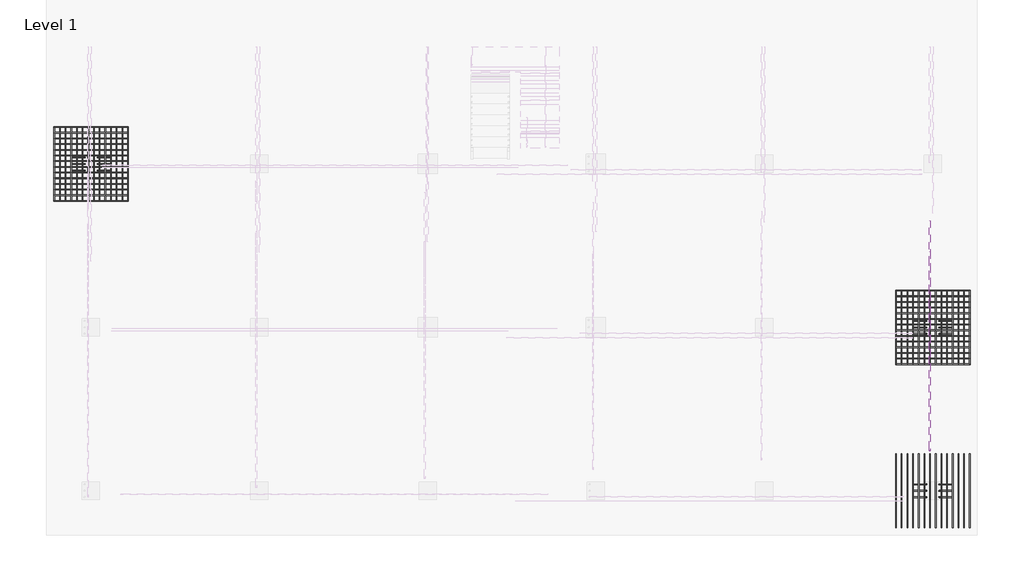
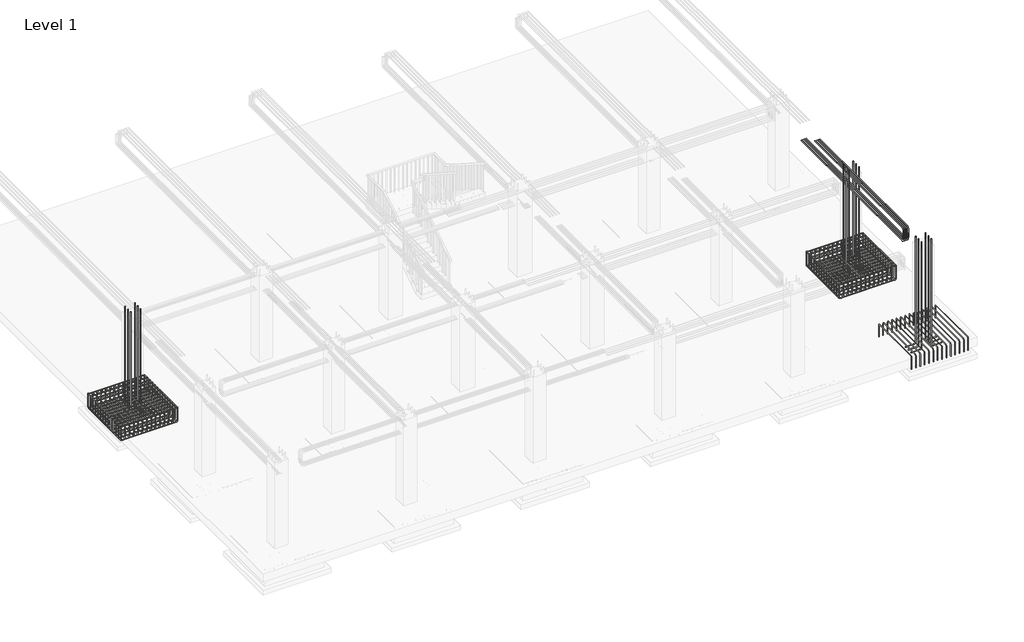
# One storey, part 8 of 17: 19 reinforcing bars.
"""IFC4 building model written with IfcOpenShell, lengths in millimetres."""

from ifc_helpers import new_model, si_unit, point, frame, origin, place, context, project, spatial, polyline, circle_curve, trimmed, segment, composite_curve, source, transform, mapped, element, save
from ifc_brep_helpers import swept_disk

model = new_model("IFC4")

# Units and contexts
model_context = context("Model", 3, world=origin())
ifc_project = project(units=[si_unit("LENGTHUNIT", "METRE", prefix="MILLI")], contexts=[model_context])

# Site, building, storey
site = spatial("IfcSite", under=ifc_project)
building = spatial("IfcBuilding", under=site)
storey = spatial("IfcBuildingStorey", under=building, Name="Level 1", Elevation=0.0)

# Reinforcing bars
placement = place(None, origin())
reinforcing_bar_shape = source(origin(), model_context, "Body", "SolidModel", [
    swept_disk(composite_curve([segment(polyline([(-13686.3632003, 4853.009457, -40.0), (-13686.3632003, 4853.009457, -504.0)]), True, "CONTINUOUS"), segment(trimmed(circle_curve(frame((-13638.3632003, 4853.009457, -504.0), z_axis=(0.0, -1.0, 0.0), x_axis=(-48.0, 0.0, 0.0)), 48.0), [point((-13686.3632003, 4853.009457, -504.0))], [point((-13638.3632003, 4853.009457, -552.0))], True, "CARTESIAN"), True, "CONTINUOUS"), segment(polyline([(-13638.3632003, 4853.009457, -552.0), (-11830.3632003, 4853.009457, -552.0)]), True, "CONTINUOUS"), segment(trimmed(circle_curve(frame((-11830.3632003, 4853.009457, -504.0), z_axis=(0.0, -1.0, 0.0), x_axis=(0.0, 0.0, -48.0)), 48.0), [point((-11830.3632003, 4853.009457, -552.0))], [point((-11782.3632003, 4853.009457, -504.0))], True, "CARTESIAN"), True, "CONTINUOUS"), segment(polyline([(-11782.3632003, 4853.009457, -504.0), (-11782.3632003, 4853.009457, -40.0)]), True, "CONTINUOUS")], self_intersect=False), 8.0),
])
element("IfcReinforcingBar", 1, at=placement, inside=storey, context=model_context, shape_type="MappedRepresentation", body=[
    mapped(reinforcing_bar_shape, transform((0.0, 0.0, 0.0), x_axis=(1.0, 0.0, 0.0), y_axis=(0.0, 1.0, 0.0), z_axis=(0.0, 0.0, 1.0))),
    mapped(reinforcing_bar_shape, transform((0.0, -146.4615385, 0.0), x_axis=(1.0, 0.0, 0.0), y_axis=(0.0, 1.0, 0.0), z_axis=(0.0, 0.0, 1.0))),
    mapped(reinforcing_bar_shape, transform((0.0, -292.9230769, 0.0), x_axis=(1.0, 0.0, 0.0), y_axis=(0.0, 1.0, 0.0), z_axis=(0.0, 0.0, 1.0))),
    mapped(reinforcing_bar_shape, transform((0.0, -439.3846154, 0.0), x_axis=(1.0, 0.0, 0.0), y_axis=(0.0, 1.0, 0.0), z_axis=(0.0, 0.0, 1.0))),
    mapped(reinforcing_bar_shape, transform((0.0, -585.8461538, 0.0), x_axis=(1.0, 0.0, 0.0), y_axis=(0.0, 1.0, 0.0), z_axis=(0.0, 0.0, 1.0))),
    mapped(reinforcing_bar_shape, transform((0.0, -732.3076923, 0.0), x_axis=(1.0, 0.0, 0.0), y_axis=(0.0, 1.0, 0.0), z_axis=(0.0, 0.0, 1.0))),
    mapped(reinforcing_bar_shape, transform((0.0, -878.7692308, 0.0), x_axis=(1.0, 0.0, 0.0), y_axis=(0.0, 1.0, 0.0), z_axis=(0.0, 0.0, 1.0))),
    mapped(reinforcing_bar_shape, transform((0.0, -1025.2307692, 0.0), x_axis=(1.0, 0.0, 0.0), y_axis=(0.0, 1.0, 0.0), z_axis=(0.0, 0.0, 1.0))),
    mapped(reinforcing_bar_shape, transform((0.0, -1171.6923077, 0.0), x_axis=(1.0, 0.0, 0.0), y_axis=(0.0, 1.0, 0.0), z_axis=(0.0, 0.0, 1.0))),
    mapped(reinforcing_bar_shape, transform((0.0, -1318.1538462, 0.0), x_axis=(1.0, 0.0, 0.0), y_axis=(0.0, 1.0, 0.0), z_axis=(0.0, 0.0, 1.0))),
    mapped(reinforcing_bar_shape, transform((0.0, -1464.6153846, 0.0), x_axis=(1.0, 0.0, 0.0), y_axis=(0.0, 1.0, 0.0), z_axis=(0.0, 0.0, 1.0))),
    mapped(reinforcing_bar_shape, transform((0.0, -1611.0769231, 0.0), x_axis=(1.0, 0.0, 0.0), y_axis=(0.0, 1.0, 0.0), z_axis=(0.0, 0.0, 1.0))),
    mapped(reinforcing_bar_shape, transform((0.0, -1757.5384615, 0.0), x_axis=(1.0, 0.0, 0.0), y_axis=(0.0, 1.0, 0.0), z_axis=(0.0, 0.0, 1.0))),
    mapped(reinforcing_bar_shape, transform((0.0, -1904.0, 0.0), x_axis=(1.0, 0.0, 0.0), y_axis=(0.0, 1.0, 0.0), z_axis=(0.0, 0.0, 1.0))),
])
reinforcing_bar_2_shape = source(origin(), model_context, "Body", "SolidModel", [
    swept_disk(composite_curve([segment(polyline([(-13686.3632003, 2949.009457, -504.0), (-13686.3632003, 2949.009457, -96.0)]), True, "CONTINUOUS"), segment(trimmed(circle_curve(frame((-13638.3632003, 2949.009457, -96.0), z_axis=(0.0, 1.0, 0.0), x_axis=(-48.0, 0.0, 0.0)), 48.0), [point((-13686.3632003, 2949.009457, -96.0))], [point((-13638.3632003, 2949.009457, -48.0))], True, "CARTESIAN"), True, "CONTINUOUS"), segment(polyline([(-13638.3632003, 2949.009457, -48.0), (-11830.3632003, 2949.009457, -48.0)]), True, "CONTINUOUS"), segment(trimmed(circle_curve(frame((-11830.3632003, 2949.009457, -96.0), z_axis=(0.0, 1.0, 0.0), x_axis=(0.0, 0.0, 48.0)), 48.0), [point((-11830.3632003, 2949.009457, -48.0))], [point((-11782.3632003, 2949.009457, -96.0))], True, "CARTESIAN"), True, "CONTINUOUS"), segment(polyline([(-11782.3632003, 2949.009457, -96.0), (-11782.3632003, 2949.009457, -504.0)]), True, "CONTINUOUS")], self_intersect=False), 8.0),
])
element("IfcReinforcingBar", 2, at=placement, inside=storey, context=model_context, shape_type="MappedRepresentation", body=[
    mapped(reinforcing_bar_2_shape, transform((0.0, 0.0, 0.0), x_axis=(1.0, 0.0, 0.0), y_axis=(0.0, 1.0, 0.0), z_axis=(0.0, 0.0, 1.0))),
    mapped(reinforcing_bar_2_shape, transform((0.0, 146.4615385, 0.0), x_axis=(1.0, 0.0, 0.0), y_axis=(0.0, 1.0, 0.0), z_axis=(0.0, 0.0, 1.0))),
    mapped(reinforcing_bar_2_shape, transform((0.0, 292.9230769, 0.0), x_axis=(1.0, 0.0, 0.0), y_axis=(0.0, 1.0, 0.0), z_axis=(0.0, 0.0, 1.0))),
    mapped(reinforcing_bar_2_shape, transform((0.0, 439.3846154, 0.0), x_axis=(1.0, 0.0, 0.0), y_axis=(0.0, 1.0, 0.0), z_axis=(0.0, 0.0, 1.0))),
    mapped(reinforcing_bar_2_shape, transform((0.0, 585.8461538, 0.0), x_axis=(1.0, 0.0, 0.0), y_axis=(0.0, 1.0, 0.0), z_axis=(0.0, 0.0, 1.0))),
    mapped(reinforcing_bar_2_shape, transform((0.0, 732.3076923, 0.0), x_axis=(1.0, 0.0, 0.0), y_axis=(0.0, 1.0, 0.0), z_axis=(0.0, 0.0, 1.0))),
    mapped(reinforcing_bar_2_shape, transform((0.0, 878.7692308, 0.0), x_axis=(1.0, 0.0, 0.0), y_axis=(0.0, 1.0, 0.0), z_axis=(0.0, 0.0, 1.0))),
    mapped(reinforcing_bar_2_shape, transform((0.0, 1025.2307692, 0.0), x_axis=(1.0, 0.0, 0.0), y_axis=(0.0, 1.0, 0.0), z_axis=(0.0, 0.0, 1.0))),
    mapped(reinforcing_bar_2_shape, transform((0.0, 1171.6923077, 0.0), x_axis=(1.0, 0.0, 0.0), y_axis=(0.0, 1.0, 0.0), z_axis=(0.0, 0.0, 1.0))),
    mapped(reinforcing_bar_2_shape, transform((0.0, 1318.1538462, 0.0), x_axis=(1.0, 0.0, 0.0), y_axis=(0.0, 1.0, 0.0), z_axis=(0.0, 0.0, 1.0))),
    mapped(reinforcing_bar_2_shape, transform((0.0, 1464.6153846, 0.0), x_axis=(1.0, 0.0, 0.0), y_axis=(0.0, 1.0, 0.0), z_axis=(0.0, 0.0, 1.0))),
    mapped(reinforcing_bar_2_shape, transform((0.0, 1611.0769231, 0.0), x_axis=(1.0, 0.0, 0.0), y_axis=(0.0, 1.0, 0.0), z_axis=(0.0, 0.0, 1.0))),
    mapped(reinforcing_bar_2_shape, transform((0.0, 1757.5384615, 0.0), x_axis=(1.0, 0.0, 0.0), y_axis=(0.0, 1.0, 0.0), z_axis=(0.0, 0.0, 1.0))),
    mapped(reinforcing_bar_2_shape, transform((0.0, 1904.0, 0.0), x_axis=(1.0, 0.0, 0.0), y_axis=(0.0, 1.0, 0.0), z_axis=(0.0, 0.0, 1.0))),
])
reinforcing_bar_3_shape = source(origin(), model_context, "Body", "SolidModel", [
    swept_disk(composite_curve([segment(polyline([(-11782.3632003, 4853.009457, -96.0), (-11782.3632003, 4853.009457, -504.0)]), True, "CONTINUOUS"), segment(trimmed(circle_curve(frame((-11782.3632003, 4805.009457, -504.0), z_axis=(-1.0, 0.0, 0.0), x_axis=(0.0, 48.0, 0.0)), 48.0), [point((-11782.3632003, 4853.009457, -504.0))], [point((-11782.3632003, 4805.009457, -552.0))], True, "CARTESIAN"), True, "CONTINUOUS"), segment(polyline([(-11782.3632003, 4805.009457, -552.0), (-11782.3632003, 2997.009457, -552.0)]), True, "CONTINUOUS"), segment(trimmed(circle_curve(frame((-11782.3632003, 2997.009457, -504.0), z_axis=(-1.0, 0.0, 0.0), x_axis=(0.0, 0.0, -48.0)), 48.0), [point((-11782.3632003, 2997.009457, -552.0))], [point((-11782.3632003, 2949.009457, -504.0))], True, "CARTESIAN"), True, "CONTINUOUS"), segment(polyline([(-11782.3632003, 2949.009457, -504.0), (-11782.3632003, 2949.009457, -96.0)]), True, "CONTINUOUS")], self_intersect=False), 8.0),
])
element("IfcReinforcingBar", 3, at=placement, inside=storey, context=model_context, shape_type="MappedRepresentation", body=[
    mapped(reinforcing_bar_3_shape, transform((0.0, 0.0, 0.0), x_axis=(1.0, 0.0, 0.0), y_axis=(0.0, 1.0, 0.0), z_axis=(0.0, 0.0, 1.0))),
    mapped(reinforcing_bar_3_shape, transform((-146.4615385, 0.0, 0.0), x_axis=(1.0, 0.0, 0.0), y_axis=(0.0, 1.0, 0.0), z_axis=(0.0, 0.0, 1.0))),
    mapped(reinforcing_bar_3_shape, transform((-292.9230769, 0.0, 0.0), x_axis=(1.0, 0.0, 0.0), y_axis=(0.0, 1.0, 0.0), z_axis=(0.0, 0.0, 1.0))),
    mapped(reinforcing_bar_3_shape, transform((-439.3846154, 0.0, 0.0), x_axis=(1.0, 0.0, 0.0), y_axis=(0.0, 1.0, 0.0), z_axis=(0.0, 0.0, 1.0))),
    mapped(reinforcing_bar_3_shape, transform((-585.8461538, 0.0, 0.0), x_axis=(1.0, 0.0, 0.0), y_axis=(0.0, 1.0, 0.0), z_axis=(0.0, 0.0, 1.0))),
    mapped(reinforcing_bar_3_shape, transform((-732.3076923, 0.0, 0.0), x_axis=(1.0, 0.0, 0.0), y_axis=(0.0, 1.0, 0.0), z_axis=(0.0, 0.0, 1.0))),
    mapped(reinforcing_bar_3_shape, transform((-878.7692308, 0.0, 0.0), x_axis=(1.0, 0.0, 0.0), y_axis=(0.0, 1.0, 0.0), z_axis=(0.0, 0.0, 1.0))),
    mapped(reinforcing_bar_3_shape, transform((-1025.2307692, 0.0, 0.0), x_axis=(1.0, 0.0, 0.0), y_axis=(0.0, 1.0, 0.0), z_axis=(0.0, 0.0, 1.0))),
    mapped(reinforcing_bar_3_shape, transform((-1171.6923077, 0.0, 0.0), x_axis=(1.0, 0.0, 0.0), y_axis=(0.0, 1.0, 0.0), z_axis=(0.0, 0.0, 1.0))),
    mapped(reinforcing_bar_3_shape, transform((-1318.1538462, 0.0, 0.0), x_axis=(1.0, 0.0, 0.0), y_axis=(0.0, 1.0, 0.0), z_axis=(0.0, 0.0, 1.0))),
    mapped(reinforcing_bar_3_shape, transform((-1464.6153846, 0.0, 0.0), x_axis=(1.0, 0.0, 0.0), y_axis=(0.0, 1.0, 0.0), z_axis=(0.0, 0.0, 1.0))),
    mapped(reinforcing_bar_3_shape, transform((-1611.0769231, 0.0, 0.0), x_axis=(1.0, 0.0, 0.0), y_axis=(0.0, 1.0, 0.0), z_axis=(0.0, 0.0, 1.0))),
    mapped(reinforcing_bar_3_shape, transform((-1757.5384615, 0.0, 0.0), x_axis=(1.0, 0.0, 0.0), y_axis=(0.0, 1.0, 0.0), z_axis=(0.0, 0.0, 1.0))),
    mapped(reinforcing_bar_3_shape, transform((-1904.0, 0.0, 0.0), x_axis=(1.0, 0.0, 0.0), y_axis=(0.0, 1.0, 0.0), z_axis=(0.0, 0.0, 1.0))),
])
reinforcing_bar_4_shape = source(origin(), model_context, "Body", "SolidModel", [
    swept_disk(composite_curve([segment(polyline([(-13686.3632003, 4853.009457, -504.0), (-13686.3632003, 4853.009457, -96.0)]), True, "CONTINUOUS"), segment(trimmed(circle_curve(frame((-13686.3632003, 4805.009457, -96.0), z_axis=(1.0, 0.0, 0.0), x_axis=(0.0, 48.0, 0.0)), 48.0), [point((-13686.3632003, 4853.009457, -96.0))], [point((-13686.3632003, 4805.009457, -48.0))], True, "CARTESIAN"), True, "CONTINUOUS"), segment(polyline([(-13686.3632003, 4805.009457, -48.0), (-13686.3632003, 2997.009457, -48.0)]), True, "CONTINUOUS"), segment(trimmed(circle_curve(frame((-13686.3632003, 2997.009457, -96.0), z_axis=(1.0, 0.0, 0.0), x_axis=(0.0, 0.0, 48.0)), 48.0), [point((-13686.3632003, 2997.009457, -48.0))], [point((-13686.3632003, 2949.009457, -96.0))], True, "CARTESIAN"), True, "CONTINUOUS"), segment(polyline([(-13686.3632003, 2949.009457, -96.0), (-13686.3632003, 2949.009457, -504.0)]), True, "CONTINUOUS")], self_intersect=False), 8.0),
])
element("IfcReinforcingBar", 4, at=placement, inside=storey, context=model_context, shape_type="MappedRepresentation", body=[
    mapped(reinforcing_bar_4_shape, transform((0.0, 0.0, 0.0), x_axis=(1.0, 0.0, 0.0), y_axis=(0.0, 1.0, 0.0), z_axis=(0.0, 0.0, 1.0))),
    mapped(reinforcing_bar_4_shape, transform((146.4615385, 0.0, 0.0), x_axis=(1.0, 0.0, 0.0), y_axis=(0.0, 1.0, 0.0), z_axis=(0.0, 0.0, 1.0))),
    mapped(reinforcing_bar_4_shape, transform((292.9230769, 0.0, 0.0), x_axis=(1.0, 0.0, 0.0), y_axis=(0.0, 1.0, 0.0), z_axis=(0.0, 0.0, 1.0))),
    mapped(reinforcing_bar_4_shape, transform((439.3846154, 0.0, 0.0), x_axis=(1.0, 0.0, 0.0), y_axis=(0.0, 1.0, 0.0), z_axis=(0.0, 0.0, 1.0))),
    mapped(reinforcing_bar_4_shape, transform((585.8461538, 0.0, 0.0), x_axis=(1.0, 0.0, 0.0), y_axis=(0.0, 1.0, 0.0), z_axis=(0.0, 0.0, 1.0))),
    mapped(reinforcing_bar_4_shape, transform((732.3076923, 0.0, 0.0), x_axis=(1.0, 0.0, 0.0), y_axis=(0.0, 1.0, 0.0), z_axis=(0.0, 0.0, 1.0))),
    mapped(reinforcing_bar_4_shape, transform((878.7692308, 0.0, 0.0), x_axis=(1.0, 0.0, 0.0), y_axis=(0.0, 1.0, 0.0), z_axis=(0.0, 0.0, 1.0))),
    mapped(reinforcing_bar_4_shape, transform((1025.2307692, 0.0, 0.0), x_axis=(1.0, 0.0, 0.0), y_axis=(0.0, 1.0, 0.0), z_axis=(0.0, 0.0, 1.0))),
    mapped(reinforcing_bar_4_shape, transform((1171.6923077, 0.0, 0.0), x_axis=(1.0, 0.0, 0.0), y_axis=(0.0, 1.0, 0.0), z_axis=(0.0, 0.0, 1.0))),
    mapped(reinforcing_bar_4_shape, transform((1318.1538462, 0.0, 0.0), x_axis=(1.0, 0.0, 0.0), y_axis=(0.0, 1.0, 0.0), z_axis=(0.0, 0.0, 1.0))),
    mapped(reinforcing_bar_4_shape, transform((1464.6153846, 0.0, 0.0), x_axis=(1.0, 0.0, 0.0), y_axis=(0.0, 1.0, 0.0), z_axis=(0.0, 0.0, 1.0))),
    mapped(reinforcing_bar_4_shape, transform((1611.0769231, 0.0, 0.0), x_axis=(1.0, 0.0, 0.0), y_axis=(0.0, 1.0, 0.0), z_axis=(0.0, 0.0, 1.0))),
    mapped(reinforcing_bar_4_shape, transform((1757.5384615, 0.0, 0.0), x_axis=(1.0, 0.0, 0.0), y_axis=(0.0, 1.0, 0.0), z_axis=(0.0, 0.0, 1.0))),
    mapped(reinforcing_bar_4_shape, transform((1904.0, 0.0, 0.0), x_axis=(1.0, 0.0, 0.0), y_axis=(0.0, 1.0, 0.0), z_axis=(0.0, 0.0, 1.0))),
])
reinforcing_bar_5_shape = source(origin(), model_context, "Body", "SolidModel", [
    swept_disk(composite_curve([segment(polyline([(-13246.9785849, 4066.509457, -550.0), (-12949.8632003, 4066.509457, -550.0)]), True, "CONTINUOUS"), segment(trimmed(circle_curve(frame((-12949.8632003, 4066.509457, -500.0), z_axis=(0.0, -1.0, 0.0), x_axis=(0.0, 0.0, -50.0)), 50.0), [point((-12949.8632003, 4066.509457, -550.0))], [point((-12899.8632003, 4066.509457, -500.0))], True, "CARTESIAN"), True, "CONTINUOUS"), segment(polyline([(-12899.8632003, 4066.509457, -500.0), (-12899.8632003, 4066.509457, 3260.0)]), True, "CONTINUOUS")], self_intersect=False), 10.0),
])
element("IfcReinforcingBar", 5, at=placement, inside=storey, context=model_context, shape_type="MappedRepresentation", body=[
    mapped(reinforcing_bar_5_shape, transform((0.0, 0.0, 0.0), x_axis=(1.0, 0.0, 0.0), y_axis=(0.0, 1.0, 0.0), z_axis=(0.0, 0.0, 1.0))),
    mapped(reinforcing_bar_5_shape, transform((0.0, -165.5, 0.0), x_axis=(1.0, 0.0, 0.0), y_axis=(0.0, 1.0, 0.0), z_axis=(0.0, 0.0, 1.0))),
    mapped(reinforcing_bar_5_shape, transform((0.0, -331.0, 0.0), x_axis=(1.0, 0.0, 0.0), y_axis=(0.0, 1.0, 0.0), z_axis=(0.0, 0.0, 1.0))),
])
reinforcing_bar_6_shape = source(origin(), model_context, "Body", "SolidModel", [
    swept_disk(composite_curve([segment(polyline([(-12221.7478157, 3735.509457, -550.0), (-12518.8632003, 3735.509457, -550.0)]), True, "CONTINUOUS"), segment(trimmed(circle_curve(frame((-12518.8632003, 3735.509457, -500.0), z_axis=(0.0, 1.0, 0.0), x_axis=(0.0, 0.0, -50.0)), 50.0), [point((-12518.8632003, 3735.509457, -550.0))], [point((-12568.8632003, 3735.509457, -500.0))], True, "CARTESIAN"), True, "CONTINUOUS"), segment(polyline([(-12568.8632003, 3735.509457, -500.0), (-12568.8632003, 3735.509457, 3260.0)]), True, "CONTINUOUS")], self_intersect=False), 10.0),
])
element("IfcReinforcingBar", 6, at=placement, inside=storey, context=model_context, shape_type="MappedRepresentation", body=[
    mapped(reinforcing_bar_6_shape, transform((0.0, 0.0, 0.0), x_axis=(1.0, 0.0, 0.0), y_axis=(0.0, 1.0, 0.0), z_axis=(0.0, 0.0, 1.0))),
    mapped(reinforcing_bar_6_shape, transform((0.0, 165.5, 0.0), x_axis=(1.0, 0.0, 0.0), y_axis=(0.0, 1.0, 0.0), z_axis=(0.0, 0.0, 1.0))),
    mapped(reinforcing_bar_6_shape, transform((0.0, 331.0, 0.0), x_axis=(1.0, 0.0, 0.0), y_axis=(0.0, 1.0, 0.0), z_axis=(0.0, 0.0, 1.0))),
])
reinforcing_bar_7_shape = source(origin(), model_context, "Body", "SolidModel", [
    swept_disk(composite_curve([segment(polyline([(8038.6367997, 636.009457, -40.0), (8038.6367997, 636.009457, -504.0)]), True, "CONTINUOUS"), segment(trimmed(circle_curve(frame((8086.6367997, 636.009457, -504.0), z_axis=(0.0, -1.0, 0.0), x_axis=(-48.0, 0.0, 0.0)), 48.0), [point((8038.6367997, 636.009457, -504.0))], [point((8086.6367997, 636.009457, -552.0))], True, "CARTESIAN"), True, "CONTINUOUS"), segment(polyline([(8086.6367997, 636.009457, -552.0), (9894.6367997, 636.009457, -552.0)]), True, "CONTINUOUS"), segment(trimmed(circle_curve(frame((9894.6367997, 636.009457, -504.0), z_axis=(0.0, -1.0, 0.0), x_axis=(0.0, 0.0, -48.0)), 48.0), [point((9894.6367997, 636.009457, -552.0))], [point((9942.6367997, 636.009457, -504.0))], True, "CARTESIAN"), True, "CONTINUOUS"), segment(polyline([(9942.6367997, 636.009457, -504.0), (9942.6367997, 636.009457, -40.0)]), True, "CONTINUOUS")], self_intersect=False), 8.0),
])
element("IfcReinforcingBar", 7, at=placement, inside=storey, context=model_context, shape_type="MappedRepresentation", body=[
    mapped(reinforcing_bar_7_shape, transform((0.0, 0.0, 0.0), x_axis=(1.0, 0.0, 0.0), y_axis=(0.0, 1.0, 0.0), z_axis=(0.0, 0.0, 1.0))),
    mapped(reinforcing_bar_7_shape, transform((0.0, -146.4615385, 0.0), x_axis=(1.0, 0.0, 0.0), y_axis=(0.0, 1.0, 0.0), z_axis=(0.0, 0.0, 1.0))),
    mapped(reinforcing_bar_7_shape, transform((0.0, -292.9230769, 0.0), x_axis=(1.0, 0.0, 0.0), y_axis=(0.0, 1.0, 0.0), z_axis=(0.0, 0.0, 1.0))),
    mapped(reinforcing_bar_7_shape, transform((0.0, -439.3846154, 0.0), x_axis=(1.0, 0.0, 0.0), y_axis=(0.0, 1.0, 0.0), z_axis=(0.0, 0.0, 1.0))),
    mapped(reinforcing_bar_7_shape, transform((0.0, -585.8461538, 0.0), x_axis=(1.0, 0.0, 0.0), y_axis=(0.0, 1.0, 0.0), z_axis=(0.0, 0.0, 1.0))),
    mapped(reinforcing_bar_7_shape, transform((0.0, -732.3076923, 0.0), x_axis=(1.0, 0.0, 0.0), y_axis=(0.0, 1.0, 0.0), z_axis=(0.0, 0.0, 1.0))),
    mapped(reinforcing_bar_7_shape, transform((0.0, -878.7692308, 0.0), x_axis=(1.0, 0.0, 0.0), y_axis=(0.0, 1.0, 0.0), z_axis=(0.0, 0.0, 1.0))),
    mapped(reinforcing_bar_7_shape, transform((0.0, -1025.2307692, 0.0), x_axis=(1.0, 0.0, 0.0), y_axis=(0.0, 1.0, 0.0), z_axis=(0.0, 0.0, 1.0))),
    mapped(reinforcing_bar_7_shape, transform((0.0, -1171.6923077, 0.0), x_axis=(1.0, 0.0, 0.0), y_axis=(0.0, 1.0, 0.0), z_axis=(0.0, 0.0, 1.0))),
    mapped(reinforcing_bar_7_shape, transform((0.0, -1318.1538462, 0.0), x_axis=(1.0, 0.0, 0.0), y_axis=(0.0, 1.0, 0.0), z_axis=(0.0, 0.0, 1.0))),
    mapped(reinforcing_bar_7_shape, transform((0.0, -1464.6153846, 0.0), x_axis=(1.0, 0.0, 0.0), y_axis=(0.0, 1.0, 0.0), z_axis=(0.0, 0.0, 1.0))),
    mapped(reinforcing_bar_7_shape, transform((0.0, -1611.0769231, 0.0), x_axis=(1.0, 0.0, 0.0), y_axis=(0.0, 1.0, 0.0), z_axis=(0.0, 0.0, 1.0))),
    mapped(reinforcing_bar_7_shape, transform((0.0, -1757.5384615, 0.0), x_axis=(1.0, 0.0, 0.0), y_axis=(0.0, 1.0, 0.0), z_axis=(0.0, 0.0, 1.0))),
    mapped(reinforcing_bar_7_shape, transform((0.0, -1904.0, 0.0), x_axis=(1.0, 0.0, 0.0), y_axis=(0.0, 1.0, 0.0), z_axis=(0.0, 0.0, 1.0))),
])
reinforcing_bar_8_shape = source(origin(), model_context, "Body", "SolidModel", [
    swept_disk(composite_curve([segment(polyline([(8038.6367997, -1267.990543, -504.0), (8038.6367997, -1267.990543, -96.0)]), True, "CONTINUOUS"), segment(trimmed(circle_curve(frame((8086.6367997, -1267.990543, -96.0), z_axis=(0.0, 1.0, 0.0), x_axis=(-48.0, 0.0, 0.0)), 48.0), [point((8038.6367997, -1267.990543, -96.0))], [point((8086.6367997, -1267.990543, -48.0))], True, "CARTESIAN"), True, "CONTINUOUS"), segment(polyline([(8086.6367997, -1267.990543, -48.0), (9894.6367997, -1267.990543, -48.0)]), True, "CONTINUOUS"), segment(trimmed(circle_curve(frame((9894.6367997, -1267.990543, -96.0), z_axis=(0.0, 1.0, 0.0), x_axis=(0.0, 0.0, 48.0)), 48.0), [point((9894.6367997, -1267.990543, -48.0))], [point((9942.6367997, -1267.990543, -96.0))], True, "CARTESIAN"), True, "CONTINUOUS"), segment(polyline([(9942.6367997, -1267.990543, -96.0), (9942.6367997, -1267.990543, -504.0)]), True, "CONTINUOUS")], self_intersect=False), 8.0),
])
element("IfcReinforcingBar", 8, at=placement, inside=storey, context=model_context, shape_type="MappedRepresentation", body=[
    mapped(reinforcing_bar_8_shape, transform((0.0, 0.0, 0.0), x_axis=(1.0, 0.0, 0.0), y_axis=(0.0, 1.0, 0.0), z_axis=(0.0, 0.0, 1.0))),
    mapped(reinforcing_bar_8_shape, transform((0.0, 146.4615385, 0.0), x_axis=(1.0, 0.0, 0.0), y_axis=(0.0, 1.0, 0.0), z_axis=(0.0, 0.0, 1.0))),
    mapped(reinforcing_bar_8_shape, transform((0.0, 292.9230769, 0.0), x_axis=(1.0, 0.0, 0.0), y_axis=(0.0, 1.0, 0.0), z_axis=(0.0, 0.0, 1.0))),
    mapped(reinforcing_bar_8_shape, transform((0.0, 439.3846154, 0.0), x_axis=(1.0, 0.0, 0.0), y_axis=(0.0, 1.0, 0.0), z_axis=(0.0, 0.0, 1.0))),
    mapped(reinforcing_bar_8_shape, transform((0.0, 585.8461538, 0.0), x_axis=(1.0, 0.0, 0.0), y_axis=(0.0, 1.0, 0.0), z_axis=(0.0, 0.0, 1.0))),
    mapped(reinforcing_bar_8_shape, transform((0.0, 732.3076923, 0.0), x_axis=(1.0, 0.0, 0.0), y_axis=(0.0, 1.0, 0.0), z_axis=(0.0, 0.0, 1.0))),
    mapped(reinforcing_bar_8_shape, transform((0.0, 878.7692308, 0.0), x_axis=(1.0, 0.0, 0.0), y_axis=(0.0, 1.0, 0.0), z_axis=(0.0, 0.0, 1.0))),
    mapped(reinforcing_bar_8_shape, transform((0.0, 1025.2307692, 0.0), x_axis=(1.0, 0.0, 0.0), y_axis=(0.0, 1.0, 0.0), z_axis=(0.0, 0.0, 1.0))),
    mapped(reinforcing_bar_8_shape, transform((0.0, 1171.6923077, 0.0), x_axis=(1.0, 0.0, 0.0), y_axis=(0.0, 1.0, 0.0), z_axis=(0.0, 0.0, 1.0))),
    mapped(reinforcing_bar_8_shape, transform((0.0, 1318.1538462, 0.0), x_axis=(1.0, 0.0, 0.0), y_axis=(0.0, 1.0, 0.0), z_axis=(0.0, 0.0, 1.0))),
    mapped(reinforcing_bar_8_shape, transform((0.0, 1464.6153846, 0.0), x_axis=(1.0, 0.0, 0.0), y_axis=(0.0, 1.0, 0.0), z_axis=(0.0, 0.0, 1.0))),
    mapped(reinforcing_bar_8_shape, transform((0.0, 1611.0769231, 0.0), x_axis=(1.0, 0.0, 0.0), y_axis=(0.0, 1.0, 0.0), z_axis=(0.0, 0.0, 1.0))),
    mapped(reinforcing_bar_8_shape, transform((0.0, 1757.5384615, 0.0), x_axis=(1.0, 0.0, 0.0), y_axis=(0.0, 1.0, 0.0), z_axis=(0.0, 0.0, 1.0))),
    mapped(reinforcing_bar_8_shape, transform((0.0, 1904.0, 0.0), x_axis=(1.0, 0.0, 0.0), y_axis=(0.0, 1.0, 0.0), z_axis=(0.0, 0.0, 1.0))),
])
reinforcing_bar_9_shape = source(origin(), model_context, "Body", "SolidModel", [
    swept_disk(composite_curve([segment(polyline([(9942.6367997, 636.009457, -96.0), (9942.6367997, 636.009457, -504.0)]), True, "CONTINUOUS"), segment(trimmed(circle_curve(frame((9942.6367997, 588.009457, -504.0), z_axis=(-1.0, 0.0, 0.0), x_axis=(0.0, 48.0, 0.0)), 48.0), [point((9942.6367997, 636.009457, -504.0))], [point((9942.6367997, 588.009457, -552.0))], True, "CARTESIAN"), True, "CONTINUOUS"), segment(polyline([(9942.6367997, 588.009457, -552.0), (9942.6367997, -1219.990543, -552.0)]), True, "CONTINUOUS"), segment(trimmed(circle_curve(frame((9942.6367997, -1219.990543, -504.0), z_axis=(-1.0, 0.0, 0.0), x_axis=(0.0, 0.0, -48.0)), 48.0), [point((9942.6367997, -1219.990543, -552.0))], [point((9942.6367997, -1267.990543, -504.0))], True, "CARTESIAN"), True, "CONTINUOUS"), segment(polyline([(9942.6367997, -1267.990543, -504.0), (9942.6367997, -1267.990543, -96.0)]), True, "CONTINUOUS")], self_intersect=False), 8.0),
])
element("IfcReinforcingBar", 9, at=placement, inside=storey, context=model_context, shape_type="MappedRepresentation", body=[
    mapped(reinforcing_bar_9_shape, transform((0.0, 0.0, 0.0), x_axis=(1.0, 0.0, 0.0), y_axis=(0.0, 1.0, 0.0), z_axis=(0.0, 0.0, 1.0))),
    mapped(reinforcing_bar_9_shape, transform((-146.4615385, 0.0, 0.0), x_axis=(1.0, 0.0, 0.0), y_axis=(0.0, 1.0, 0.0), z_axis=(0.0, 0.0, 1.0))),
    mapped(reinforcing_bar_9_shape, transform((-292.9230769, 0.0, 0.0), x_axis=(1.0, 0.0, 0.0), y_axis=(0.0, 1.0, 0.0), z_axis=(0.0, 0.0, 1.0))),
    mapped(reinforcing_bar_9_shape, transform((-439.3846154, 0.0, 0.0), x_axis=(1.0, 0.0, 0.0), y_axis=(0.0, 1.0, 0.0), z_axis=(0.0, 0.0, 1.0))),
    mapped(reinforcing_bar_9_shape, transform((-585.8461538, 0.0, 0.0), x_axis=(1.0, 0.0, 0.0), y_axis=(0.0, 1.0, 0.0), z_axis=(0.0, 0.0, 1.0))),
    mapped(reinforcing_bar_9_shape, transform((-732.3076923, 0.0, 0.0), x_axis=(1.0, 0.0, 0.0), y_axis=(0.0, 1.0, 0.0), z_axis=(0.0, 0.0, 1.0))),
    mapped(reinforcing_bar_9_shape, transform((-878.7692308, 0.0, 0.0), x_axis=(1.0, 0.0, 0.0), y_axis=(0.0, 1.0, 0.0), z_axis=(0.0, 0.0, 1.0))),
    mapped(reinforcing_bar_9_shape, transform((-1025.2307692, 0.0, 0.0), x_axis=(1.0, 0.0, 0.0), y_axis=(0.0, 1.0, 0.0), z_axis=(0.0, 0.0, 1.0))),
    mapped(reinforcing_bar_9_shape, transform((-1171.6923077, 0.0, 0.0), x_axis=(1.0, 0.0, 0.0), y_axis=(0.0, 1.0, 0.0), z_axis=(0.0, 0.0, 1.0))),
    mapped(reinforcing_bar_9_shape, transform((-1318.1538462, 0.0, 0.0), x_axis=(1.0, 0.0, 0.0), y_axis=(0.0, 1.0, 0.0), z_axis=(0.0, 0.0, 1.0))),
    mapped(reinforcing_bar_9_shape, transform((-1464.6153846, 0.0, 0.0), x_axis=(1.0, 0.0, 0.0), y_axis=(0.0, 1.0, 0.0), z_axis=(0.0, 0.0, 1.0))),
    mapped(reinforcing_bar_9_shape, transform((-1611.0769231, 0.0, 0.0), x_axis=(1.0, 0.0, 0.0), y_axis=(0.0, 1.0, 0.0), z_axis=(0.0, 0.0, 1.0))),
    mapped(reinforcing_bar_9_shape, transform((-1757.5384615, 0.0, 0.0), x_axis=(1.0, 0.0, 0.0), y_axis=(0.0, 1.0, 0.0), z_axis=(0.0, 0.0, 1.0))),
    mapped(reinforcing_bar_9_shape, transform((-1904.0, 0.0, 0.0), x_axis=(1.0, 0.0, 0.0), y_axis=(0.0, 1.0, 0.0), z_axis=(0.0, 0.0, 1.0))),
])
reinforcing_bar_10_shape = source(origin(), model_context, "Body", "SolidModel", [
    swept_disk(composite_curve([segment(polyline([(8038.6367997, 636.009457, -504.0), (8038.6367997, 636.009457, -96.0)]), True, "CONTINUOUS"), segment(trimmed(circle_curve(frame((8038.6367997, 588.009457, -96.0), z_axis=(1.0, 0.0, 0.0), x_axis=(0.0, 48.0, 0.0)), 48.0), [point((8038.6367997, 636.009457, -96.0))], [point((8038.6367997, 588.009457, -48.0))], True, "CARTESIAN"), True, "CONTINUOUS"), segment(polyline([(8038.6367997, 588.009457, -48.0), (8038.6367997, -1219.990543, -48.0)]), True, "CONTINUOUS"), segment(trimmed(circle_curve(frame((8038.6367997, -1219.990543, -96.0), z_axis=(1.0, 0.0, 0.0), x_axis=(0.0, 0.0, 48.0)), 48.0), [point((8038.6367997, -1219.990543, -48.0))], [point((8038.6367997, -1267.990543, -96.0))], True, "CARTESIAN"), True, "CONTINUOUS"), segment(polyline([(8038.6367997, -1267.990543, -96.0), (8038.6367997, -1267.990543, -504.0)]), True, "CONTINUOUS")], self_intersect=False), 8.0),
])
element("IfcReinforcingBar", 10, at=placement, inside=storey, context=model_context, shape_type="MappedRepresentation", body=[
    mapped(reinforcing_bar_10_shape, transform((0.0, 0.0, 0.0), x_axis=(1.0, 0.0, 0.0), y_axis=(0.0, 1.0, 0.0), z_axis=(0.0, 0.0, 1.0))),
    mapped(reinforcing_bar_10_shape, transform((146.4615385, 0.0, 0.0), x_axis=(1.0, 0.0, 0.0), y_axis=(0.0, 1.0, 0.0), z_axis=(0.0, 0.0, 1.0))),
    mapped(reinforcing_bar_10_shape, transform((292.9230769, 0.0, 0.0), x_axis=(1.0, 0.0, 0.0), y_axis=(0.0, 1.0, 0.0), z_axis=(0.0, 0.0, 1.0))),
    mapped(reinforcing_bar_10_shape, transform((439.3846154, 0.0, 0.0), x_axis=(1.0, 0.0, 0.0), y_axis=(0.0, 1.0, 0.0), z_axis=(0.0, 0.0, 1.0))),
    mapped(reinforcing_bar_10_shape, transform((585.8461538, 0.0, 0.0), x_axis=(1.0, 0.0, 0.0), y_axis=(0.0, 1.0, 0.0), z_axis=(0.0, 0.0, 1.0))),
    mapped(reinforcing_bar_10_shape, transform((732.3076923, 0.0, 0.0), x_axis=(1.0, 0.0, 0.0), y_axis=(0.0, 1.0, 0.0), z_axis=(0.0, 0.0, 1.0))),
    mapped(reinforcing_bar_10_shape, transform((878.7692308, 0.0, 0.0), x_axis=(1.0, 0.0, 0.0), y_axis=(0.0, 1.0, 0.0), z_axis=(0.0, 0.0, 1.0))),
    mapped(reinforcing_bar_10_shape, transform((1025.2307692, 0.0, 0.0), x_axis=(1.0, 0.0, 0.0), y_axis=(0.0, 1.0, 0.0), z_axis=(0.0, 0.0, 1.0))),
    mapped(reinforcing_bar_10_shape, transform((1171.6923077, 0.0, 0.0), x_axis=(1.0, 0.0, 0.0), y_axis=(0.0, 1.0, 0.0), z_axis=(0.0, 0.0, 1.0))),
    mapped(reinforcing_bar_10_shape, transform((1318.1538462, 0.0, 0.0), x_axis=(1.0, 0.0, 0.0), y_axis=(0.0, 1.0, 0.0), z_axis=(0.0, 0.0, 1.0))),
    mapped(reinforcing_bar_10_shape, transform((1464.6153846, 0.0, 0.0), x_axis=(1.0, 0.0, 0.0), y_axis=(0.0, 1.0, 0.0), z_axis=(0.0, 0.0, 1.0))),
    mapped(reinforcing_bar_10_shape, transform((1611.0769231, 0.0, 0.0), x_axis=(1.0, 0.0, 0.0), y_axis=(0.0, 1.0, 0.0), z_axis=(0.0, 0.0, 1.0))),
    mapped(reinforcing_bar_10_shape, transform((1757.5384615, 0.0, 0.0), x_axis=(1.0, 0.0, 0.0), y_axis=(0.0, 1.0, 0.0), z_axis=(0.0, 0.0, 1.0))),
    mapped(reinforcing_bar_10_shape, transform((1904.0, 0.0, 0.0), x_axis=(1.0, 0.0, 0.0), y_axis=(0.0, 1.0, 0.0), z_axis=(0.0, 0.0, 1.0))),
])
reinforcing_bar_11_shape = source(origin(), model_context, "Body", "SolidModel", [
    swept_disk(composite_curve([segment(polyline([(8478.0214151, -150.490543, -550.0), (8775.1367997, -150.490543, -550.0)]), True, "CONTINUOUS"), segment(trimmed(circle_curve(frame((8775.1367997, -150.490543, -500.0), z_axis=(0.0, -1.0, 0.0), x_axis=(0.0, 0.0, -50.0)), 50.0), [point((8775.1367997, -150.490543, -550.0))], [point((8825.1367997, -150.490543, -500.0))], True, "CARTESIAN"), True, "CONTINUOUS"), segment(polyline([(8825.1367997, -150.490543, -500.0), (8825.1367997, -150.490543, 3260.0)]), True, "CONTINUOUS")], self_intersect=False), 10.0),
])
element("IfcReinforcingBar", 11, at=placement, inside=storey, context=model_context, shape_type="MappedRepresentation", body=[
    mapped(reinforcing_bar_11_shape, transform((0.0, 0.0, 0.0), x_axis=(1.0, 0.0, 0.0), y_axis=(0.0, 1.0, 0.0), z_axis=(0.0, 0.0, 1.0))),
    mapped(reinforcing_bar_11_shape, transform((0.0, -165.5, 0.0), x_axis=(1.0, 0.0, 0.0), y_axis=(0.0, 1.0, 0.0), z_axis=(0.0, 0.0, 1.0))),
    mapped(reinforcing_bar_11_shape, transform((0.0, -331.0, 0.0), x_axis=(1.0, 0.0, 0.0), y_axis=(0.0, 1.0, 0.0), z_axis=(0.0, 0.0, 1.0))),
])
reinforcing_bar_12_shape = source(origin(), model_context, "Body", "SolidModel", [
    swept_disk(composite_curve([segment(polyline([(9503.2521843, -481.490543, -550.0), (9206.1367997, -481.490543, -550.0)]), True, "CONTINUOUS"), segment(trimmed(circle_curve(frame((9206.1367997, -481.490543, -500.0), z_axis=(0.0, 1.0, 0.0), x_axis=(0.0, 0.0, -50.0)), 50.0), [point((9206.1367997, -481.490543, -550.0))], [point((9156.1367997, -481.490543, -500.0))], True, "CARTESIAN"), True, "CONTINUOUS"), segment(polyline([(9156.1367997, -481.490543, -500.0), (9156.1367997, -481.490543, 3260.0)]), True, "CONTINUOUS")], self_intersect=False), 10.0),
])
element("IfcReinforcingBar", 12, at=placement, inside=storey, context=model_context, shape_type="MappedRepresentation", body=[
    mapped(reinforcing_bar_12_shape, transform((0.0, 0.0, 0.0), x_axis=(1.0, 0.0, 0.0), y_axis=(0.0, 1.0, 0.0), z_axis=(0.0, 0.0, 1.0))),
    mapped(reinforcing_bar_12_shape, transform((0.0, 165.5, 0.0), x_axis=(1.0, 0.0, 0.0), y_axis=(0.0, 1.0, 0.0), z_axis=(0.0, 0.0, 1.0))),
    mapped(reinforcing_bar_12_shape, transform((0.0, 331.0, 0.0), x_axis=(1.0, 0.0, 0.0), y_axis=(0.0, 1.0, 0.0), z_axis=(0.0, 0.0, 1.0))),
])
reinforcing_bar_13_shape = source(origin(), model_context, "Body", "SolidModel", [
    swept_disk(composite_curve([segment(polyline([(8038.6367997, -3580.990543, -504.0), (8038.6367997, -3580.990543, -96.0)]), True, "CONTINUOUS"), segment(trimmed(circle_curve(frame((8038.6367997, -3628.990543, -96.0), z_axis=(1.0, 0.0, 0.0), x_axis=(0.0, 48.0, 0.0)), 48.0), [point((8038.6367997, -3580.990543, -96.0))], [point((8038.6367997, -3628.990543, -48.0))], True, "CARTESIAN"), True, "CONTINUOUS"), segment(polyline([(8038.6367997, -3628.990543, -48.0), (8038.6367997, -5436.990543, -48.0)]), True, "CONTINUOUS"), segment(trimmed(circle_curve(frame((8038.6367997, -5436.990543, -96.0), z_axis=(1.0, 0.0, 0.0), x_axis=(0.0, 0.0, 48.0)), 48.0), [point((8038.6367997, -5436.990543, -48.0))], [point((8038.6367997, -5484.990543, -96.0))], True, "CARTESIAN"), True, "CONTINUOUS"), segment(polyline([(8038.6367997, -5484.990543, -96.0), (8038.6367997, -5484.990543, -504.0)]), True, "CONTINUOUS")], self_intersect=False), 8.0),
])
element("IfcReinforcingBar", 13, at=placement, inside=storey, context=model_context, shape_type="MappedRepresentation", body=[
    mapped(reinforcing_bar_13_shape, transform((0.0, 0.0, 0.0), x_axis=(1.0, 0.0, 0.0), y_axis=(0.0, 1.0, 0.0), z_axis=(0.0, 0.0, 1.0))),
    mapped(reinforcing_bar_13_shape, transform((146.4615385, 0.0, 0.0), x_axis=(1.0, 0.0, 0.0), y_axis=(0.0, 1.0, 0.0), z_axis=(0.0, 0.0, 1.0))),
    mapped(reinforcing_bar_13_shape, transform((292.9230769, 0.0, 0.0), x_axis=(1.0, 0.0, 0.0), y_axis=(0.0, 1.0, 0.0), z_axis=(0.0, 0.0, 1.0))),
    mapped(reinforcing_bar_13_shape, transform((439.3846154, 0.0, 0.0), x_axis=(1.0, 0.0, 0.0), y_axis=(0.0, 1.0, 0.0), z_axis=(0.0, 0.0, 1.0))),
    mapped(reinforcing_bar_13_shape, transform((585.8461538, 0.0, 0.0), x_axis=(1.0, 0.0, 0.0), y_axis=(0.0, 1.0, 0.0), z_axis=(0.0, 0.0, 1.0))),
    mapped(reinforcing_bar_13_shape, transform((732.3076923, 0.0, 0.0), x_axis=(1.0, 0.0, 0.0), y_axis=(0.0, 1.0, 0.0), z_axis=(0.0, 0.0, 1.0))),
    mapped(reinforcing_bar_13_shape, transform((878.7692308, 0.0, 0.0), x_axis=(1.0, 0.0, 0.0), y_axis=(0.0, 1.0, 0.0), z_axis=(0.0, 0.0, 1.0))),
    mapped(reinforcing_bar_13_shape, transform((1025.2307692, 0.0, 0.0), x_axis=(1.0, 0.0, 0.0), y_axis=(0.0, 1.0, 0.0), z_axis=(0.0, 0.0, 1.0))),
    mapped(reinforcing_bar_13_shape, transform((1171.6923077, 0.0, 0.0), x_axis=(1.0, 0.0, 0.0), y_axis=(0.0, 1.0, 0.0), z_axis=(0.0, 0.0, 1.0))),
    mapped(reinforcing_bar_13_shape, transform((1318.1538462, 0.0, 0.0), x_axis=(1.0, 0.0, 0.0), y_axis=(0.0, 1.0, 0.0), z_axis=(0.0, 0.0, 1.0))),
    mapped(reinforcing_bar_13_shape, transform((1464.6153846, 0.0, 0.0), x_axis=(1.0, 0.0, 0.0), y_axis=(0.0, 1.0, 0.0), z_axis=(0.0, 0.0, 1.0))),
    mapped(reinforcing_bar_13_shape, transform((1611.0769231, 0.0, 0.0), x_axis=(1.0, 0.0, 0.0), y_axis=(0.0, 1.0, 0.0), z_axis=(0.0, 0.0, 1.0))),
    mapped(reinforcing_bar_13_shape, transform((1757.5384615, 0.0, 0.0), x_axis=(1.0, 0.0, 0.0), y_axis=(0.0, 1.0, 0.0), z_axis=(0.0, 0.0, 1.0))),
    mapped(reinforcing_bar_13_shape, transform((1904.0, 0.0, 0.0), x_axis=(1.0, 0.0, 0.0), y_axis=(0.0, 1.0, 0.0), z_axis=(0.0, 0.0, 1.0))),
])
reinforcing_bar_14_shape = source(origin(), model_context, "Body", "SolidModel", [
    swept_disk(composite_curve([segment(polyline([(8478.0214151, -4367.490543, -550.0), (8775.1367997, -4367.490543, -550.0)]), True, "CONTINUOUS"), segment(trimmed(circle_curve(frame((8775.1367997, -4367.490543, -500.0), z_axis=(0.0, -1.0, 0.0), x_axis=(0.0, 0.0, -50.0)), 50.0), [point((8775.1367997, -4367.490543, -550.0))], [point((8825.1367997, -4367.490543, -500.0))], True, "CARTESIAN"), True, "CONTINUOUS"), segment(polyline([(8825.1367997, -4367.490543, -500.0), (8825.1367997, -4367.490543, 3260.0)]), True, "CONTINUOUS")], self_intersect=False), 10.0),
])
element("IfcReinforcingBar", 14, at=placement, inside=storey, context=model_context, shape_type="MappedRepresentation", body=[
    mapped(reinforcing_bar_14_shape, transform((0.0, 0.0, 0.0), x_axis=(1.0, 0.0, 0.0), y_axis=(0.0, 1.0, 0.0), z_axis=(0.0, 0.0, 1.0))),
    mapped(reinforcing_bar_14_shape, transform((0.0, -165.5, 0.0), x_axis=(1.0, 0.0, 0.0), y_axis=(0.0, 1.0, 0.0), z_axis=(0.0, 0.0, 1.0))),
    mapped(reinforcing_bar_14_shape, transform((0.0, -331.0, 0.0), x_axis=(1.0, 0.0, 0.0), y_axis=(0.0, 1.0, 0.0), z_axis=(0.0, 0.0, 1.0))),
])
reinforcing_bar_15_shape = source(origin(), model_context, "Body", "SolidModel", [
    swept_disk(composite_curve([segment(polyline([(9503.2521843, -4698.490543, -550.0), (9206.1367997, -4698.490543, -550.0)]), True, "CONTINUOUS"), segment(trimmed(circle_curve(frame((9206.1367997, -4698.490543, -500.0), z_axis=(0.0, 1.0, 0.0), x_axis=(0.0, 0.0, -50.0)), 50.0), [point((9206.1367997, -4698.490543, -550.0))], [point((9156.1367997, -4698.490543, -500.0))], True, "CARTESIAN"), True, "CONTINUOUS"), segment(polyline([(9156.1367997, -4698.490543, -500.0), (9156.1367997, -4698.490543, 3260.0)]), True, "CONTINUOUS")], self_intersect=False), 10.0),
])
element("IfcReinforcingBar", 15, at=placement, inside=storey, context=model_context, shape_type="MappedRepresentation", body=[
    mapped(reinforcing_bar_15_shape, transform((0.0, 0.0, 0.0), x_axis=(1.0, 0.0, 0.0), y_axis=(0.0, 1.0, 0.0), z_axis=(0.0, 0.0, 1.0))),
    mapped(reinforcing_bar_15_shape, transform((0.0, 165.5, 0.0), x_axis=(1.0, 0.0, 0.0), y_axis=(0.0, 1.0, 0.0), z_axis=(0.0, 0.0, 1.0))),
    mapped(reinforcing_bar_15_shape, transform((0.0, 331.0, 0.0), x_axis=(1.0, 0.0, 0.0), y_axis=(0.0, 1.0, 0.0), z_axis=(0.0, 0.0, 1.0))),
])
reinforcing_bar_16_shape = source(origin(), model_context, "Body", "SolidModel", [
    swept_disk(composite_curve([segment(polyline([(9070.6367997, 2437.509457, 2518.0), (9070.6367997, -3444.490543, 2518.0)]), True, "CONTINUOUS"), segment(trimmed(circle_curve(frame((9070.6367997, -3444.490543, 2568.0), z_axis=(-1.0, 0.0, 0.0), x_axis=(0.0, 0.0, -50.0)), 50.0), [point((9070.6367997, -3444.490543, 2518.0))], [point((9070.6367997, -3494.490543, 2568.0))], True, "CARTESIAN"), True, "CONTINUOUS"), segment(polyline([(9070.6367997, -3494.490543, 2568.0), (9070.6367997, -3494.490543, 2748.0)]), True, "CONTINUOUS")], self_intersect=False), 10.0),
])
element("IfcReinforcingBar", 16, at=placement, inside=storey, context=model_context, shape_type="MappedRepresentation", body=[
    mapped(reinforcing_bar_16_shape, transform((0.0, 0.0, 0.0), x_axis=(1.0, 0.0, 0.0), y_axis=(0.0, 1.0, 0.0), z_axis=(0.0, 0.0, 1.0))),
    mapped(reinforcing_bar_16_shape, transform((-53.3333333, 0.0, 0.0), x_axis=(1.0, 0.0, 0.0), y_axis=(0.0, 1.0, 0.0), z_axis=(0.0, 0.0, 1.0))),
    mapped(reinforcing_bar_16_shape, transform((-106.6666667, 0.0, 0.0), x_axis=(1.0, 0.0, 0.0), y_axis=(0.0, 1.0, 0.0), z_axis=(0.0, 0.0, 1.0))),
    mapped(reinforcing_bar_16_shape, transform((-160.0, 0.0, 0.0), x_axis=(1.0, 0.0, 0.0), y_axis=(0.0, 1.0, 0.0), z_axis=(0.0, 0.0, 1.0))),
])
reinforcing_bar_17_shape = source(origin(), model_context, "Body", "SolidModel", [
    swept_disk(composite_curve([segment(polyline([(8910.6367997, 1637.909457, 2978.0), (8910.6367997, -3449.990543, 2978.0)]), True, "CONTINUOUS"), segment(trimmed(circle_curve(frame((8910.6367997, -3449.990543, 2928.0), z_axis=(1.0, 0.0, 0.0), x_axis=(0.0, 0.0, 50.0)), 50.0), [point((8910.6367997, -3449.990543, 2978.0))], [point((8910.6367997, -3499.990543, 2928.0))], True, "CARTESIAN"), True, "CONTINUOUS"), segment(polyline([(8910.6367997, -3499.990543, 2928.0), (8910.6367997, -3499.990543, 2608.0)]), True, "CONTINUOUS")], self_intersect=False), 10.0),
])
element("IfcReinforcingBar", 17, at=placement, inside=storey, context=model_context, shape_type="MappedRepresentation", body=[
    mapped(reinforcing_bar_17_shape, transform((0.0, 0.0, 0.0), x_axis=(1.0, 0.0, 0.0), y_axis=(0.0, 1.0, 0.0), z_axis=(0.0, 0.0, 1.0))),
    mapped(reinforcing_bar_17_shape, transform((53.3333333, 0.0, 0.0), x_axis=(1.0, 0.0, 0.0), y_axis=(0.0, 1.0, 0.0), z_axis=(0.0, 0.0, 1.0))),
    mapped(reinforcing_bar_17_shape, transform((106.6666667, 0.0, 0.0), x_axis=(1.0, 0.0, 0.0), y_axis=(0.0, 1.0, 0.0), z_axis=(0.0, 0.0, 1.0))),
    mapped(reinforcing_bar_17_shape, transform((160.0, 0.0, 0.0), x_axis=(1.0, 0.0, 0.0), y_axis=(0.0, 1.0, 0.0), z_axis=(0.0, 0.0, 1.0))),
])
reinforcing_bar_18_shape = source(origin(), model_context, "Body", "SolidModel", [
    swept_disk(composite_curve([segment(polyline([(9070.6367997, 2437.509457, 2518.0), (9070.6367997, -3444.490543, 2518.0)]), True, "CONTINUOUS"), segment(trimmed(circle_curve(frame((9070.6367997, -3444.490543, 2568.0), z_axis=(-1.0, 0.0, 0.0), x_axis=(0.0, 0.0, -50.0)), 50.0), [point((9070.6367997, -3444.490543, 2518.0))], [point((9070.6367997, -3494.490543, 2568.0))], True, "CARTESIAN"), True, "CONTINUOUS"), segment(polyline([(9070.6367997, -3494.490543, 2568.0), (9070.6367997, -3494.490543, 2748.0)]), True, "CONTINUOUS")], self_intersect=False), 10.0),
])
element("IfcReinforcingBar", 18, at=placement, inside=storey, context=model_context, shape_type="MappedRepresentation", body=[
    mapped(reinforcing_bar_18_shape, transform((0.0, 0.0, 0.0), x_axis=(1.0, 0.0, 0.0), y_axis=(0.0, 1.0, 0.0), z_axis=(0.0, 0.0, 1.0))),
    mapped(reinforcing_bar_18_shape, transform((-53.3333333, 0.0, 0.0), x_axis=(1.0, 0.0, 0.0), y_axis=(0.0, 1.0, 0.0), z_axis=(0.0, 0.0, 1.0))),
    mapped(reinforcing_bar_18_shape, transform((-106.6666667, 0.0, 0.0), x_axis=(1.0, 0.0, 0.0), y_axis=(0.0, 1.0, 0.0), z_axis=(0.0, 0.0, 1.0))),
    mapped(reinforcing_bar_18_shape, transform((-160.0, 0.0, 0.0), x_axis=(1.0, 0.0, 0.0), y_axis=(0.0, 1.0, 0.0), z_axis=(0.0, 0.0, 1.0))),
])
reinforcing_bar_19_shape = source(origin(), model_context, "Body", "SolidModel", [
    swept_disk(composite_curve([segment(polyline([(8910.6367997, 1637.909457, 2978.0), (8910.6367997, -3449.990543, 2978.0)]), True, "CONTINUOUS"), segment(trimmed(circle_curve(frame((8910.6367997, -3449.990543, 2928.0), z_axis=(1.0, 0.0, 0.0), x_axis=(0.0, 0.0, 50.0)), 50.0), [point((8910.6367997, -3449.990543, 2978.0))], [point((8910.6367997, -3499.990543, 2928.0))], True, "CARTESIAN"), True, "CONTINUOUS"), segment(polyline([(8910.6367997, -3499.990543, 2928.0), (8910.6367997, -3499.990543, 2608.0)]), True, "CONTINUOUS")], self_intersect=False), 10.0),
])
element("IfcReinforcingBar", 19, at=placement, inside=storey, context=model_context, shape_type="MappedRepresentation", body=[
    mapped(reinforcing_bar_19_shape, transform((0.0, 0.0, 0.0), x_axis=(1.0, 0.0, 0.0), y_axis=(0.0, 1.0, 0.0), z_axis=(0.0, 0.0, 1.0))),
    mapped(reinforcing_bar_19_shape, transform((53.3333333, 0.0, 0.0), x_axis=(1.0, 0.0, 0.0), y_axis=(0.0, 1.0, 0.0), z_axis=(0.0, 0.0, 1.0))),
    mapped(reinforcing_bar_19_shape, transform((106.6666667, 0.0, 0.0), x_axis=(1.0, 0.0, 0.0), y_axis=(0.0, 1.0, 0.0), z_axis=(0.0, 0.0, 1.0))),
    mapped(reinforcing_bar_19_shape, transform((160.0, 0.0, 0.0), x_axis=(1.0, 0.0, 0.0), y_axis=(0.0, 1.0, 0.0), z_axis=(0.0, 0.0, 1.0))),
])

save(model, "model.ifc")

# Revit data of these elements
# Elements 1, 2, 3, 4, 5, 6, 7, 8, 9, 10, 11, 12, 13, 14, 15, 16, 17, 18, 19 (IfcReinforcingBar)
#   Phase Created = New Construction
